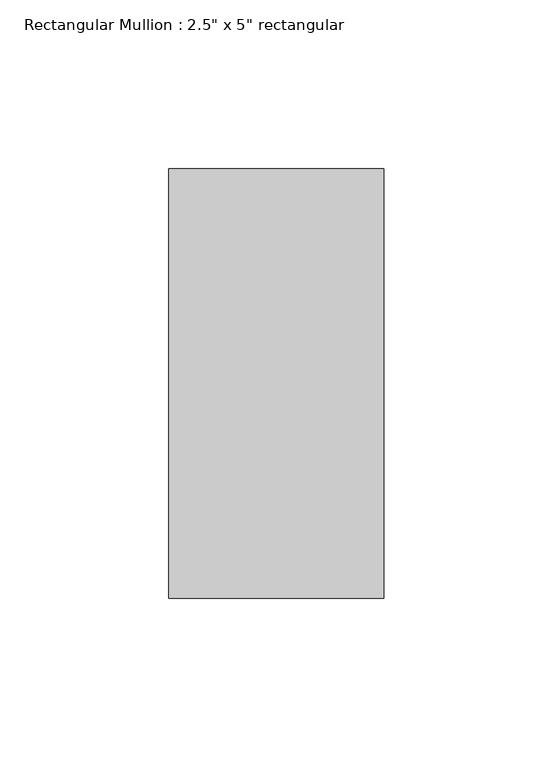
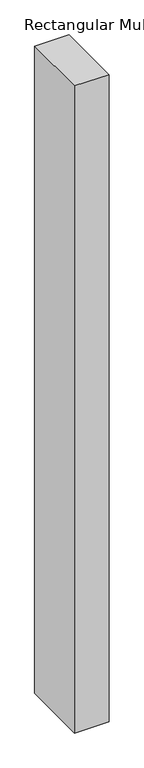
"""IFC4 building model written with IfcOpenShell, lengths in millimetres: member geometry."""

from ifc_helpers import new_model, si_unit, frame, origin, place, context, project, spatial, polyline, outline, extrude, source, transform, mapped, element, save


def member_bcb6a316(model_context):
    return source(origin(), model_context, "Body", "SweptSolid", [
        extrude(outline(polyline([(0.0, 63.5), (0.0, -63.5), (-63.5, -63.5), (-63.5, 63.5), (0.0, 63.5)])), frame((0.0, 0.0, -1257.3), z_axis=(0.0, 0.0, 1.0), x_axis=(1.0, 0.0, 0.0)), (0.0, 0.0, 1.0), 1257.3),
    ])


if __name__ == "__main__":
    model = new_model("IFC4")
    model_context = context("Model", 3, world=origin())
    ifc_project = project(units=[si_unit("LENGTHUNIT", "METRE", prefix="MILLI")], contexts=[model_context])
    site = spatial("IfcSite", under=ifc_project)
    building = spatial("IfcBuilding", under=site)
    placement = place(None, origin())
    member_shape = member_bcb6a316(model_context)
    element("IfcMember", 1, ObjectType="Rectangular Mullion : 2.5\" x 5\" rectangular", at=placement, inside=building, context=model_context, shape_type="MappedRepresentation", body=[
        mapped(member_shape, transform((0.0, 0.0, 0.0), x_axis=(1.0, 0.0, 0.0), y_axis=(0.0, 1.0, 0.0), z_axis=(0.0, 0.0, 1.0))),
    ])
    save(model, "model.ifc")

# Revit data of these elements
# Type "Rectangular Mullion : 2.5\" x 5\" rectangular"
#   built-in parameter 1007304 = 0.416667 (stored number, unit not read)
#   built-in parameter 1007301 = 0.104167 (stored number, unit not read)
#   built-in parameter 1007300 = 0.104167 (stored number, unit not read)
# Element 1 (IfcMember, "Rectangular Mullion : 2.5\" x 5\" rectangular")
#   Materials on its faces: "Iron, Ductile"
# Materials
#   "Iron, Ductile": class "Metal", colour RGB 0 0 0, transparency 0, Description = "Ductile cast iron", Cost = 0
